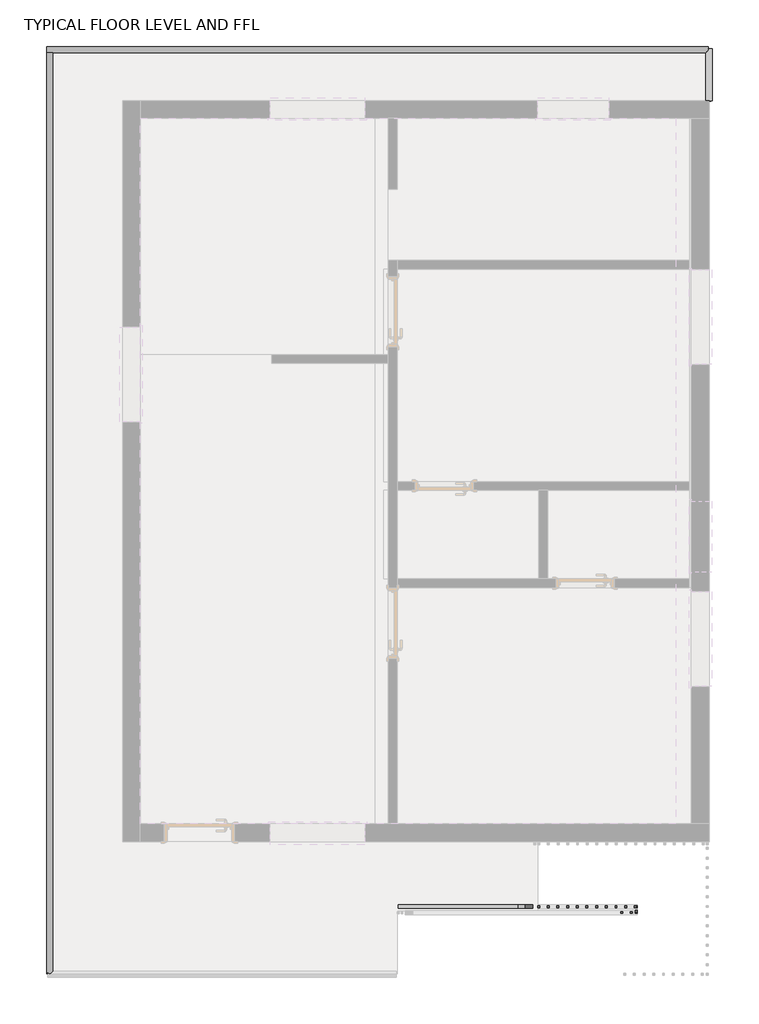
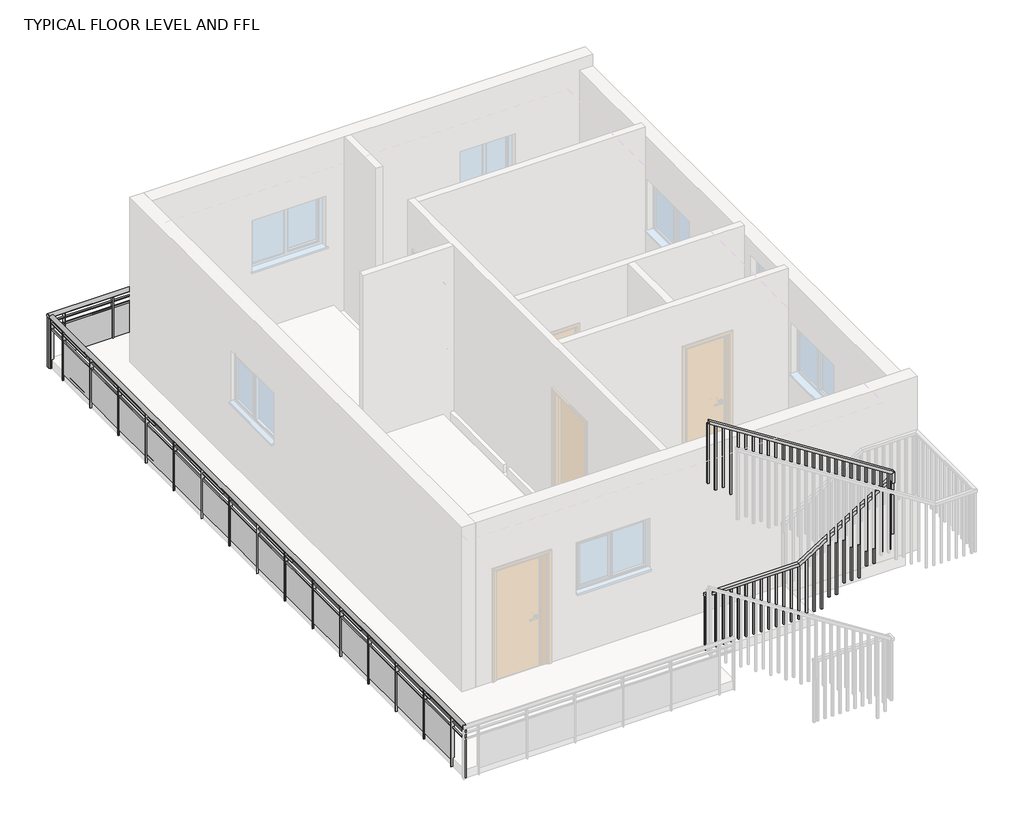
# One storey, part 3 of 3: 4 railings.
"""IFC4 building model written with IfcOpenShell, lengths in millimetres."""

from ifc_helpers import new_model, si_unit, point, frame, origin, place, context, project, spatial, polyline, ellipse_curve, trimmed, outline, extrude, faceted_brep, element, save
from ifc_brep_helpers import plane_surface, extruded_surface, advanced_brep

model = new_model("IFC4")

# Units and contexts
model_context = context("Model", 3, world=origin())
ifc_project = project(units=[si_unit("LENGTHUNIT", "METRE", prefix="MILLI")], contexts=[model_context])

# Site, building, storey
site = spatial("IfcSite", under=ifc_project)
building = spatial("IfcBuilding", under=site)
storey = spatial("IfcBuildingStorey", under=building, Name="TYPICAL FLOOR LEVEL AND FFL", Elevation=3535.68)

# Railings
placement = place(None, origin())
element("IfcRailing", 1, ObjectType="1100mm", at=placement, inside=storey, context=model_context, shape_type="SolidModel", body=[
    faceted_brep([(-10483.549573, -11032.9255223, 4676.32), (-10483.549573, -11032.9255223, 4626.32), (-10483.549573, -11082.9255223, 4626.32), (-10483.549573, -11082.9255223, 4676.32), (-8934.2055614, -11032.9255223, 4676.32), (-8919.5781391, -11032.9255223, 4626.32), (-8919.5781391, -11082.9255223, 4626.32), (-8934.2055614, -11082.9255223, 4676.32), (-7435.149573, -11032.9255223, 5635.5044027), (-7435.149573, -11082.9255223, 5635.5044027), (-7435.149573, -11082.9255223, 5576.1449155), (-7435.149573, -11032.9255223, 5576.1449155)], [[[0, 1, 2, 3]], [[1, 0, 4, 5]], [[2, 1, 5, 6]], [[3, 2, 6, 7]], [[0, 3, 7, 4]], [[8, 9, 10, 11]], [[5, 4, 8, 11]], [[6, 5, 11, 10]], [[7, 6, 10, 9]], [[4, 7, 9, 8]]]),
    faceted_brep([(-7385.149573, -11032.9255223, 5651.68), (-7385.149573, -11032.9255223, 5601.68), (-7435.149573, -11032.9255223, 5601.68), (-7435.149573, -11032.9255223, 5651.68), (-7385.149573, -11109.5255223, 5651.68), (-7435.149573, -11109.5255223, 5651.68), (-7435.149573, -11159.5255223, 5601.68), (-7385.149573, -11159.5255223, 5601.68)], [[[0, 1, 2, 3]], [[4, 5, 6, 7]], [[1, 0, 4, 7]], [[2, 1, 7, 6]], [[3, 2, 6, 5]], [[0, 3, 5, 4]]]),
    faceted_brep([(-7385.149573, -11109.5255223, 5651.68), (-7385.149573, -11159.5255223, 5601.68), (-7435.149573, -11159.5255223, 5601.68), (-7435.149573, -11109.5255223, 5651.68), (-7385.149573, -11109.5255223, 5798.3802481), (-7435.149573, -11109.5255223, 5771.0172146), (-7435.149573, -11159.5255223, 5771.0172146), (-7385.149573, -11159.5255223, 5798.3802481)], [[[0, 1, 2, 3]], [[4, 5, 6, 7]], [[1, 0, 4, 7]], [[2, 1, 7, 6]], [[3, 2, 6, 5]], [[0, 3, 5, 4]]]),
    faceted_brep([(-7385.149573, -11159.5255223, 5798.3802481), (-7435.149573, -11159.5255223, 5771.0172146), (-7435.149573, -11109.5255223, 5771.0172146), (-7385.149573, -11109.5255223, 5798.3802481), (-10457.8773536, -11159.5255223, 7764.96), (-10457.8773536, -11109.5255223, 7764.96), (-10457.8773536, -11109.5255223, 7705.5964137), (-10457.8773536, -11159.5255223, 7705.5964137)], [[[0, 1, 2, 3]], [[4, 5, 6, 7]], [[1, 0, 4, 7]], [[2, 1, 7, 6]], [[3, 2, 6, 5]], [[0, 3, 5, 4]]]),
    extrude(outline(polyline([(6664.96, -10460.149573), (7707.0506592, -10460.149573), (7723.0509356, -10485.149573), (6664.96, -10485.149573), (6664.96, -10460.149573)])), frame((0.0, -11147.0255223, 0.0), z_axis=(0.0, 1.0, 0.0), x_axis=(0.0, 0.0, 1.0)), (0.0, 0.0, 1.0), 25.0),
    extrude(outline(polyline([(6502.4, -10335.149573), (7627.0492772, -10335.149573), (7643.0495536, -10360.149573), (6502.4, -10360.149573), (6502.4, -10335.149573)])), frame((0.0, -11147.0255223, 0.0), z_axis=(0.0, 1.0, 0.0), x_axis=(0.0, 0.0, 1.0)), (0.0, 0.0, 1.0), 25.0),
    extrude(outline(polyline([(6502.4, -10210.149573), (7547.0478952, -10210.149573), (7563.0481716, -10235.149573), (6502.4, -10235.149573), (6502.4, -10210.149573)])), frame((0.0, -11147.0255223, 0.0), z_axis=(0.0, 1.0, 0.0), x_axis=(0.0, 0.0, 1.0)), (0.0, 0.0, 1.0), 25.0),
    extrude(outline(polyline([(6339.84, -10085.149573), (7467.0465132, -10085.149573), (7483.0467896, -10110.149573), (6339.84, -10110.149573), (6339.84, -10085.149573)])), frame((0.0, -11147.0255223, 0.0), z_axis=(0.0, 1.0, 0.0), x_axis=(0.0, 0.0, 1.0)), (0.0, 0.0, 1.0), 25.0),
    extrude(outline(polyline([(6339.84, -9960.149573), (7387.0451312, -9960.149573), (7403.0454076, -9985.149573), (6339.84, -9985.149573), (6339.84, -9960.149573)])), frame((0.0, -11147.0255223, 0.0), z_axis=(0.0, 1.0, 0.0), x_axis=(0.0, 0.0, 1.0)), (0.0, 0.0, 1.0), 25.0),
    extrude(outline(polyline([(6177.28, -9835.149573), (7307.0437492, -9835.149573), (7323.0440256, -9860.149573), (6177.28, -9860.149573), (6177.28, -9835.149573)])), frame((0.0, -11147.0255223, 0.0), z_axis=(0.0, 1.0, 0.0), x_axis=(0.0, 0.0, 1.0)), (0.0, 0.0, 1.0), 25.0),
    extrude(outline(polyline([(6177.28, -9710.149573), (7227.0423672, -9710.149573), (7243.0426436, -9735.149573), (6177.28, -9735.149573), (6177.28, -9710.149573)])), frame((0.0, -11147.0255223, 0.0), z_axis=(0.0, 1.0, 0.0), x_axis=(0.0, 0.0, 1.0)), (0.0, 0.0, 1.0), 25.0),
    extrude(outline(polyline([(6014.72, -9585.149573), (7147.0409852, -9585.149573), (7163.0412616, -9610.149573), (6014.72, -9610.149573), (6014.72, -9585.149573)])), frame((0.0, -11147.0255223, 0.0), z_axis=(0.0, 1.0, 0.0), x_axis=(0.0, 0.0, 1.0)), (0.0, 0.0, 1.0), 25.0),
    extrude(outline(polyline([(6014.72, -9460.149573), (7067.0396031, -9460.149573), (7083.0398795, -9485.149573), (6014.72, -9485.149573), (6014.72, -9460.149573)])), frame((0.0, -11147.0255223, 0.0), z_axis=(0.0, 1.0, 0.0), x_axis=(0.0, 0.0, 1.0)), (0.0, 0.0, 1.0), 25.0),
    extrude(outline(polyline([(5852.16, -9335.149573), (6987.0382211, -9335.149573), (7003.0384975, -9360.149573), (5852.16, -9360.149573), (5852.16, -9335.149573)])), frame((0.0, -11147.0255223, 0.0), z_axis=(0.0, 1.0, 0.0), x_axis=(0.0, 0.0, 1.0)), (0.0, 0.0, 1.0), 25.0),
    extrude(outline(polyline([(5852.16, -9210.149573), (6907.0368391, -9210.149573), (6923.0371155, -9235.149573), (5852.16, -9235.149573), (5852.16, -9210.149573)])), frame((0.0, -11147.0255223, 0.0), z_axis=(0.0, 1.0, 0.0), x_axis=(0.0, 0.0, 1.0)), (0.0, 0.0, 1.0), 25.0),
    extrude(outline(polyline([(5689.6, -9085.149573), (6827.0354571, -9085.149573), (6843.0357335, -9110.149573), (5689.6, -9110.149573), (5689.6, -9085.149573)])), frame((0.0, -11147.0255223, 0.0), z_axis=(0.0, 1.0, 0.0), x_axis=(0.0, 0.0, 1.0)), (0.0, 0.0, 1.0), 25.0),
    extrude(outline(polyline([(5689.6, -8960.149573), (6747.0340751, -8960.149573), (6763.0343515, -8985.149573), (5689.6, -8985.149573), (5689.6, -8960.149573)])), frame((0.0, -11147.0255223, 0.0), z_axis=(0.0, 1.0, 0.0), x_axis=(0.0, 0.0, 1.0)), (0.0, 0.0, 1.0), 25.0),
    extrude(outline(polyline([(5527.04, -8835.149573), (6667.0326931, -8835.149573), (6683.0329695, -8860.149573), (5527.04, -8860.149573), (5527.04, -8835.149573)])), frame((0.0, -11147.0255223, 0.0), z_axis=(0.0, 1.0, 0.0), x_axis=(0.0, 0.0, 1.0)), (0.0, 0.0, 1.0), 25.0),
    extrude(outline(polyline([(5527.04, -8710.149573), (6587.0313111, -8710.149573), (6603.0315875, -8735.149573), (5527.04, -8735.149573), (5527.04, -8710.149573)])), frame((0.0, -11147.0255223, 0.0), z_axis=(0.0, 1.0, 0.0), x_axis=(0.0, 0.0, 1.0)), (0.0, 0.0, 1.0), 25.0),
    extrude(outline(polyline([(5364.48, -8585.149573), (6507.0299291, -8585.149573), (6523.0302055, -8610.149573), (5364.48, -8610.149573), (5364.48, -8585.149573)])), frame((0.0, -11147.0255223, 0.0), z_axis=(0.0, 1.0, 0.0), x_axis=(0.0, 0.0, 1.0)), (0.0, 0.0, 1.0), 25.0),
    extrude(outline(polyline([(5364.48, -8460.149573), (6427.0285471, -8460.149573), (6443.0288235, -8485.149573), (5364.48, -8485.149573), (5364.48, -8460.149573)])), frame((0.0, -11147.0255223, 0.0), z_axis=(0.0, 1.0, 0.0), x_axis=(0.0, 0.0, 1.0)), (0.0, 0.0, 1.0), 25.0),
    extrude(outline(polyline([(5201.92, -8335.149573), (6347.0271651, -8335.149573), (6363.0274415, -8360.149573), (5201.92, -8360.149573), (5201.92, -8335.149573)])), frame((0.0, -11147.0255223, 0.0), z_axis=(0.0, 1.0, 0.0), x_axis=(0.0, 0.0, 1.0)), (0.0, 0.0, 1.0), 25.0),
    extrude(outline(polyline([(5201.92, -8210.149573), (6267.0257831, -8210.149573), (6283.0260595, -8235.149573), (5201.92, -8235.149573), (5201.92, -8210.149573)])), frame((0.0, -11147.0255223, 0.0), z_axis=(0.0, 1.0, 0.0), x_axis=(0.0, 0.0, 1.0)), (0.0, 0.0, 1.0), 25.0),
    extrude(outline(polyline([(5039.36, -8085.149573), (6187.024401, -8085.149573), (6203.0246774, -8110.149573), (5039.36, -8110.149573), (5039.36, -8085.149573)])), frame((0.0, -11147.0255223, 0.0), z_axis=(0.0, 1.0, 0.0), x_axis=(0.0, 0.0, 1.0)), (0.0, 0.0, 1.0), 25.0),
    extrude(outline(polyline([(5039.36, -7960.149573), (6107.023019, -7960.149573), (6123.0232954, -7985.149573), (5039.36, -7985.149573), (5039.36, -7960.149573)])), frame((0.0, -11147.0255223, 0.0), z_axis=(0.0, 1.0, 0.0), x_axis=(0.0, 0.0, 1.0)), (0.0, 0.0, 1.0), 25.0),
    extrude(outline(polyline([(4876.8, -7835.149573), (6027.021637, -7835.149573), (6043.0219134, -7860.149573), (4876.8, -7860.149573), (4876.8, -7835.149573)])), frame((0.0, -11147.0255223, 0.0), z_axis=(0.0, 1.0, 0.0), x_axis=(0.0, 0.0, 1.0)), (0.0, 0.0, 1.0), 25.0),
    extrude(outline(polyline([(4876.8, -7710.149573), (5947.020255, -7710.149573), (5963.0205314, -7735.149573), (4876.8, -7735.149573), (4876.8, -7710.149573)])), frame((0.0, -11147.0255223, 0.0), z_axis=(0.0, 1.0, 0.0), x_axis=(0.0, 0.0, 1.0)), (0.0, 0.0, 1.0), 25.0),
    extrude(outline(polyline([(4714.24, -7585.149573), (5867.018873, -7585.149573), (5883.0191494, -7610.149573), (4714.24, -7610.149573), (4714.24, -7585.149573)])), frame((0.0, -11147.0255223, 0.0), z_axis=(0.0, 1.0, 0.0), x_axis=(0.0, 0.0, 1.0)), (0.0, 0.0, 1.0), 25.0),
    extrude(outline(polyline([(4714.24, -7460.149573), (5787.017491, -7460.149573), (5803.0177674, -7485.149573), (4714.24, -7485.149573), (4714.24, -7460.149573)])), frame((0.0, -11147.0255223, 0.0), z_axis=(0.0, 1.0, 0.0), x_axis=(0.0, 0.0, 1.0)), (0.0, 0.0, 1.0), 25.0),
    extrude(outline(polyline([(-7422.649573, -11107.9255223), (-7397.649573, -11107.9255223), (-7397.649573, -11132.9255223), (-7422.649573, -11132.9255223), (-7422.649573, -11107.9255223)])), frame((0.0, 0.0, 4701.5601967), z_axis=(0.0, 0.0, 1.0), x_axis=(1.0, 0.0, 0.0)), (0.0, 0.0, 1.0), 900.1198033),
    extrude(outline(polyline([(5577.1686899, -7433.549573), (4389.12, -7433.549573), (4389.12, -7408.549573), (5593.1651638, -7408.549573), (5577.1686899, -7433.549573)])), frame((0.0, -11070.4255223, 0.0), z_axis=(0.0, 1.0, 0.0), x_axis=(0.0, 0.0, 1.0)), (0.0, 0.0, 1.0), 25.0),
    extrude(outline(polyline([(5497.1863201, -7558.549573), (4389.12, -7558.549573), (4389.12, -7533.549573), (5513.1827941, -7533.549573), (5497.1863201, -7558.549573)])), frame((0.0, -11070.4255223, 0.0), z_axis=(0.0, 1.0, 0.0), x_axis=(0.0, 0.0, 1.0)), (0.0, 0.0, 1.0), 25.0),
    extrude(outline(polyline([(5417.2039504, -7683.549573), (4226.56, -7683.549573), (4226.56, -7658.549573), (5433.2004243, -7658.549573), (5417.2039504, -7683.549573)])), frame((0.0, -11070.4255223, 0.0), z_axis=(0.0, 1.0, 0.0), x_axis=(0.0, 0.0, 1.0)), (0.0, 0.0, 1.0), 25.0),
    extrude(outline(polyline([(5337.2215806, -7808.549573), (4226.56, -7808.549573), (4226.56, -7783.549573), (5353.2180546, -7783.549573), (5337.2215806, -7808.549573)])), frame((0.0, -11070.4255223, 0.0), z_axis=(0.0, 1.0, 0.0), x_axis=(0.0, 0.0, 1.0)), (0.0, 0.0, 1.0), 25.0),
    extrude(outline(polyline([(5257.2392109, -7933.549573), (4064.0, -7933.549573), (4064.0, -7908.549573), (5273.2356848, -7908.549573), (5257.2392109, -7933.549573)])), frame((0.0, -11070.4255223, 0.0), z_axis=(0.0, 1.0, 0.0), x_axis=(0.0, 0.0, 1.0)), (0.0, 0.0, 1.0), 25.0),
    extrude(outline(polyline([(5177.2568411, -8058.549573), (4064.0, -8058.549573), (4064.0, -8033.549573), (5193.2533151, -8033.549573), (5177.2568411, -8058.549573)])), frame((0.0, -11070.4255223, 0.0), z_axis=(0.0, 1.0, 0.0), x_axis=(0.0, 0.0, 1.0)), (0.0, 0.0, 1.0), 25.0),
    extrude(outline(polyline([(5097.2744714, -8183.549573), (4064.0, -8183.549573), (4064.0, -8158.549573), (5113.2709453, -8158.549573), (5097.2744714, -8183.549573)])), frame((0.0, -11070.4255223, 0.0), z_axis=(0.0, 1.0, 0.0), x_axis=(0.0, 0.0, 1.0)), (0.0, 0.0, 1.0), 25.0),
    extrude(outline(polyline([(5017.2921016, -8308.549573), (3901.44, -8308.549573), (3901.44, -8283.549573), (5033.2885756, -8283.549573), (5017.2921016, -8308.549573)])), frame((0.0, -11070.4255223, 0.0), z_axis=(0.0, 1.0, 0.0), x_axis=(0.0, 0.0, 1.0)), (0.0, 0.0, 1.0), 25.0),
    extrude(outline(polyline([(4937.3097319, -8433.549573), (3901.44, -8433.549573), (3901.44, -8408.549573), (4953.3062058, -8408.549573), (4937.3097319, -8433.549573)])), frame((0.0, -11070.4255223, 0.0), z_axis=(0.0, 1.0, 0.0), x_axis=(0.0, 0.0, 1.0)), (0.0, 0.0, 1.0), 25.0),
    extrude(outline(polyline([(4857.3273621, -8558.549573), (3738.88, -8558.549573), (3738.88, -8533.549573), (4873.3238361, -8533.549573), (4857.3273621, -8558.549573)])), frame((0.0, -11070.4255223, 0.0), z_axis=(0.0, 1.0, 0.0), x_axis=(0.0, 0.0, 1.0)), (0.0, 0.0, 1.0), 25.0),
    extrude(outline(polyline([(4777.3449924, -8683.549573), (3738.88, -8683.549573), (3738.88, -8658.549573), (4793.3414663, -8658.549573), (4777.3449924, -8683.549573)])), frame((0.0, -11070.4255223, 0.0), z_axis=(0.0, 1.0, 0.0), x_axis=(0.0, 0.0, 1.0)), (0.0, 0.0, 1.0), 25.0),
    extrude(outline(polyline([(4697.3626226, -8808.549573), (3664.7203468, -8808.549573), (3664.7203468, -8783.549573), (4713.3590966, -8783.549573), (4697.3626226, -8808.549573)])), frame((0.0, -11070.4255223, 0.0), z_axis=(0.0, 1.0, 0.0), x_axis=(0.0, 0.0, 1.0)), (0.0, 0.0, 1.0), 25.0),
    extrude(outline(polyline([(4617.3802529, -8933.549573), (3584.737977, -8933.549573), (3584.737977, -8908.549573), (4633.3767268, -8908.549573), (4617.3802529, -8933.549573)])), frame((0.0, -11070.4255223, 0.0), z_axis=(0.0, 1.0, 0.0), x_axis=(0.0, 0.0, 1.0)), (0.0, 0.0, 1.0), 25.0),
    extrude(outline(polyline([(-9058.549573, -11070.4255223), (-9058.549573, -11045.4255223), (-9033.549573, -11045.4255223), (-9033.549573, -11070.4255223), (-9058.549573, -11070.4255223)])), frame((0.0, 0.0, 3576.32), z_axis=(0.0, 0.0, 1.0), x_axis=(1.0, 0.0, 0.0)), (0.0, 0.0, 1.0), 1050.0),
    extrude(outline(polyline([(-9183.549573, -11070.4255223), (-9183.549573, -11045.4255223), (-9158.549573, -11045.4255223), (-9158.549573, -11070.4255223), (-9183.549573, -11070.4255223)])), frame((0.0, 0.0, 3576.32), z_axis=(0.0, 0.0, 1.0), x_axis=(1.0, 0.0, 0.0)), (0.0, 0.0, 1.0), 1050.0),
    extrude(outline(polyline([(-9308.549573, -11070.4255223), (-9308.549573, -11045.4255223), (-9283.549573, -11045.4255223), (-9283.549573, -11070.4255223), (-9308.549573, -11070.4255223)])), frame((0.0, 0.0, 3576.32), z_axis=(0.0, 0.0, 1.0), x_axis=(1.0, 0.0, 0.0)), (0.0, 0.0, 1.0), 1050.0),
    extrude(outline(polyline([(-9433.549573, -11070.4255223), (-9433.549573, -11045.4255223), (-9408.549573, -11045.4255223), (-9408.549573, -11070.4255223), (-9433.549573, -11070.4255223)])), frame((0.0, 0.0, 3576.32), z_axis=(0.0, 0.0, 1.0), x_axis=(1.0, 0.0, 0.0)), (0.0, 0.0, 1.0), 1050.0),
    extrude(outline(polyline([(-9558.549573, -11070.4255223), (-9558.549573, -11045.4255223), (-9533.549573, -11045.4255223), (-9533.549573, -11070.4255223), (-9558.549573, -11070.4255223)])), frame((0.0, 0.0, 3576.32), z_axis=(0.0, 0.0, 1.0), x_axis=(1.0, 0.0, 0.0)), (0.0, 0.0, 1.0), 1050.0),
    extrude(outline(polyline([(-9683.549573, -11070.4255223), (-9683.549573, -11045.4255223), (-9658.549573, -11045.4255223), (-9658.549573, -11070.4255223), (-9683.549573, -11070.4255223)])), frame((0.0, 0.0, 3576.32), z_axis=(0.0, 0.0, 1.0), x_axis=(1.0, 0.0, 0.0)), (0.0, 0.0, 1.0), 1050.0),
    extrude(outline(polyline([(-9808.549573, -11070.4255223), (-9808.549573, -11045.4255223), (-9783.549573, -11045.4255223), (-9783.549573, -11070.4255223), (-9808.549573, -11070.4255223)])), frame((0.0, 0.0, 3576.32), z_axis=(0.0, 0.0, 1.0), x_axis=(1.0, 0.0, 0.0)), (0.0, 0.0, 1.0), 1050.0),
    extrude(outline(polyline([(-9933.549573, -11070.4255223), (-9933.549573, -11045.4255223), (-9908.549573, -11045.4255223), (-9908.549573, -11070.4255223), (-9933.549573, -11070.4255223)])), frame((0.0, 0.0, 3576.32), z_axis=(0.0, 0.0, 1.0), x_axis=(1.0, 0.0, 0.0)), (0.0, 0.0, 1.0), 1050.0),
    extrude(outline(polyline([(-10058.549573, -11070.4255223), (-10058.549573, -11045.4255223), (-10033.549573, -11045.4255223), (-10033.549573, -11070.4255223), (-10058.549573, -11070.4255223)])), frame((0.0, 0.0, 3576.32), z_axis=(0.0, 0.0, 1.0), x_axis=(1.0, 0.0, 0.0)), (0.0, 0.0, 1.0), 1050.0),
    extrude(outline(polyline([(-10183.549573, -11070.4255223), (-10183.549573, -11045.4255223), (-10158.549573, -11045.4255223), (-10158.549573, -11070.4255223), (-10183.549573, -11070.4255223)])), frame((0.0, 0.0, 3576.32), z_axis=(0.0, 0.0, 1.0), x_axis=(1.0, 0.0, 0.0)), (0.0, 0.0, 1.0), 1050.0),
    extrude(outline(polyline([(-10308.549573, -11070.4255223), (-10308.549573, -11045.4255223), (-10283.549573, -11045.4255223), (-10283.549573, -11070.4255223), (-10308.549573, -11070.4255223)])), frame((0.0, 0.0, 3576.32), z_axis=(0.0, 0.0, 1.0), x_axis=(1.0, 0.0, 0.0)), (0.0, 0.0, 1.0), 1050.0),
    extrude(outline(polyline([(-10433.549573, -11070.4255223), (-10433.549573, -11045.4255223), (-10408.549573, -11045.4255223), (-10408.549573, -11070.4255223), (-10433.549573, -11070.4255223)])), frame((0.0, 0.0, 3576.32), z_axis=(0.0, 0.0, 1.0), x_axis=(1.0, 0.0, 0.0)), (0.0, 0.0, 1.0), 1050.0),
    extrude(outline(polyline([(-7422.649573, -11122.0255223), (-7397.649573, -11122.0255223), (-7397.649573, -11147.0255223), (-7422.649573, -11147.0255223), (-7422.649573, -11122.0255223)])), frame((0.0, 0.0, 4701.5601967), z_axis=(0.0, 0.0, 1.0), x_axis=(1.0, 0.0, 0.0)), (0.0, 0.0, 1.0), 900.1198033),
    extrude(outline(polyline([(5584.1431525, -7422.649573), (4389.12, -7422.649573), (4389.12, -7397.649573), (5600.1396265, -7397.649573), (5584.1431525, -7422.649573)])), frame((0.0, -11070.4255223, 0.0), z_axis=(0.0, 1.0, 0.0), x_axis=(0.0, 0.0, 1.0)), (0.0, 0.0, 1.0), 25.0),
    extrude(outline(polyline([(6664.96, -10458.549573), (7706.0266415, -10458.549573), (7722.0269179, -10483.549573), (6664.96, -10483.549573), (6664.96, -10458.549573)])), frame((0.0, -11147.0255223, 0.0), z_axis=(0.0, 1.0, 0.0), x_axis=(0.0, 0.0, 1.0)), (0.0, 0.0, 1.0), 25.0),
    extrude(outline(polyline([(-10483.549573, -11070.4255223), (-10483.549573, -11045.4255223), (-10458.549573, -11045.4255223), (-10458.549573, -11070.4255223), (-10483.549573, -11070.4255223)])), frame((0.0, 0.0, 3576.32), z_axis=(0.0, 0.0, 1.0), x_axis=(1.0, 0.0, 0.0)), (0.0, 0.0, 1.0), 1050.0),
])
element("IfcRailing", 2, ObjectType="Glass_Panel-Bottom_Fill", at=placement, inside=storey, context=model_context, shape_type="SolidModel", body=[
    advanced_brep(
    [(-15017.4420435, 42.847874, 4435.68), (-15017.4420435, -37.152126, 4435.68), (-6483.0420435, 42.847874, 4435.68), (-6483.0420435, -37.152126, 4435.68)],
    [
        (0, 1, ellipse_curve(frame((-15017.4420435, 2.847874, 4435.68), z_axis=(-1.0, 0.0, 0.0), x_axis=(0.0, -1.0, 0.0)), 40.0, 30.0)),
        (1, 0, ellipse_curve(frame((-15017.4420435, 2.847874, 4435.68), z_axis=(-1.0, 0.0, 0.0), x_axis=(0.0, -1.0, 0.0)), 40.0, 30.0)),
        (2, 3, ellipse_curve(frame((-6483.0420435, 2.847874, 4435.68), z_axis=(1.0, 0.0, 0.0), x_axis=(0.0, -1.0, 0.0)), 40.0, 30.0)),
        (3, 2, ellipse_curve(frame((-6483.0420435, 2.847874, 4435.68), z_axis=(1.0, 0.0, 0.0), x_axis=(0.0, -1.0, 0.0)), 40.0, 30.0)),
        (0, 2),
        (3, 1),
    ],
    [
        plane_surface(frame((-15017.4420435, 2.847874, 4435.68), z_axis=(-1.0, 0.0, 0.0), x_axis=(0.0, 1.0, 0.0))),
        plane_surface(frame((-6483.0420435, 2.847874, 4435.68), z_axis=(1.0, 0.0, 0.0), x_axis=(0.0, 1.0, 0.0))),
        extruded_surface(trimmed(ellipse_curve(frame((-6483.0420435, 2.847874, 4435.68), z_axis=(-1.0, 0.0, 0.0), x_axis=(0.0, -1.0, 0.0)), 40.0, 30.0), [point((-6483.0420435, 42.847874, 4435.68))], [point((-6483.0420435, -37.152126, 4435.68))], True, "CARTESIAN"), (-8534.4, 0.0, 0.0), 8534.4),
        extruded_surface(trimmed(ellipse_curve(frame((-6483.0420435, 2.847874, 4435.68), z_axis=(-1.0, 0.0, 0.0), x_axis=(0.0, -1.0, 0.0)), 40.0, 30.0), [point((-6483.0420435, -37.152126, 4435.68))], [point((-6483.0420435, 42.847874, 4435.68))], True, "CARTESIAN"), (-8534.4, 0.0, 0.0), 8534.4),
    ],
    [
        (0, [[1, 2]]),
        (1, [[3, 4]]),
        (2, [[-1, 5, -4, 6]]),
        (3, [[-2, -6, -3, -5]]),
    ],
),
    extrude(outline(polyline([(-15017.4420435, -6.5428911), (-15017.4420435, 13.4571089), (-6483.0420435, 13.4571089), (-6483.0420435, -6.5428911), (-15017.4420435, -6.5428911)])), frame((0.0, 0.0, 4315.68), z_axis=(0.0, 0.0, 1.0), x_axis=(1.0, 0.0, 0.0)), (0.0, 0.0, 1.0), 20.0),
    extrude(outline(polyline([(-15017.4420435, -6.5428911), (-15017.4420435, 13.4571089), (-6483.0420435, 13.4571089), (-6483.0420435, -6.5428911), (-15017.4420435, -6.5428911)])), frame((0.0, 0.0, 4215.68), z_axis=(0.0, 0.0, 1.0), x_axis=(1.0, 0.0, 0.0)), (0.0, 0.0, 1.0), 20.0),
    extrude(outline(polyline([(-6756.2420435, 28.4571089), (-6744.2420435, 28.4571089), (-6744.2420435, -21.5428911), (-6756.2420435, -21.5428911), (-6756.2420435, 28.4571089)])), frame((0.0, 0.0, 3535.68), z_axis=(0.0, 0.0, 1.0), x_axis=(1.0, 0.0, 0.0)), (0.0, 0.0, 1.0), 870.0),
    extrude(outline(polyline([(-7550.2420435, 1.7322988), (-6750.2420435, 1.7322988), (-6750.2420435, -3.2677012), (-7550.2420435, -3.2677012), (-7550.2420435, 1.7322988)])), frame((0.0, 0.0, 3635.68), z_axis=(0.0, 0.0, 1.0), x_axis=(1.0, 0.0, 0.0)), (0.0, 0.0, 1.0), 580.0),
    extrude(outline(polyline([(-7556.2420435, 28.4571089), (-7544.2420435, 28.4571089), (-7544.2420435, -21.5428911), (-7556.2420435, -21.5428911), (-7556.2420435, 28.4571089)])), frame((0.0, 0.0, 3535.68), z_axis=(0.0, 0.0, 1.0), x_axis=(1.0, 0.0, 0.0)), (0.0, 0.0, 1.0), 870.0),
    extrude(outline(polyline([(-8350.2420435, 1.7322988), (-7550.2420435, 1.7322988), (-7550.2420435, -3.2677012), (-8350.2420435, -3.2677012), (-8350.2420435, 1.7322988)])), frame((0.0, 0.0, 3635.68), z_axis=(0.0, 0.0, 1.0), x_axis=(1.0, 0.0, 0.0)), (0.0, 0.0, 1.0), 580.0),
    extrude(outline(polyline([(-8356.2420435, 28.4571089), (-8344.2420435, 28.4571089), (-8344.2420435, -21.5428911), (-8356.2420435, -21.5428911), (-8356.2420435, 28.4571089)])), frame((0.0, 0.0, 3535.68), z_axis=(0.0, 0.0, 1.0), x_axis=(1.0, 0.0, 0.0)), (0.0, 0.0, 1.0), 870.0),
    extrude(outline(polyline([(-9150.2420435, 1.7322988), (-8350.2420435, 1.7322988), (-8350.2420435, -3.2677012), (-9150.2420435, -3.2677012), (-9150.2420435, 1.7322988)])), frame((0.0, 0.0, 3635.68), z_axis=(0.0, 0.0, 1.0), x_axis=(1.0, 0.0, 0.0)), (0.0, 0.0, 1.0), 580.0),
    extrude(outline(polyline([(-9156.2420435, 28.4571089), (-9144.2420435, 28.4571089), (-9144.2420435, -21.5428911), (-9156.2420435, -21.5428911), (-9156.2420435, 28.4571089)])), frame((0.0, 0.0, 3535.68), z_axis=(0.0, 0.0, 1.0), x_axis=(1.0, 0.0, 0.0)), (0.0, 0.0, 1.0), 870.0),
    extrude(outline(polyline([(-9950.2420435, 1.7322988), (-9150.2420435, 1.7322988), (-9150.2420435, -3.2677012), (-9950.2420435, -3.2677012), (-9950.2420435, 1.7322988)])), frame((0.0, 0.0, 3635.68), z_axis=(0.0, 0.0, 1.0), x_axis=(1.0, 0.0, 0.0)), (0.0, 0.0, 1.0), 580.0),
    extrude(outline(polyline([(-9956.2420435, 28.4571089), (-9944.2420435, 28.4571089), (-9944.2420435, -21.5428911), (-9956.2420435, -21.5428911), (-9956.2420435, 28.4571089)])), frame((0.0, 0.0, 3535.68), z_axis=(0.0, 0.0, 1.0), x_axis=(1.0, 0.0, 0.0)), (0.0, 0.0, 1.0), 870.0),
    extrude(outline(polyline([(-10750.2420435, 1.7322988), (-9950.2420435, 1.7322988), (-9950.2420435, -3.2677012), (-10750.2420435, -3.2677012), (-10750.2420435, 1.7322988)])), frame((0.0, 0.0, 3635.68), z_axis=(0.0, 0.0, 1.0), x_axis=(1.0, 0.0, 0.0)), (0.0, 0.0, 1.0), 580.0),
    extrude(outline(polyline([(-10756.2420435, 28.4571089), (-10744.2420435, 28.4571089), (-10744.2420435, -21.5428911), (-10756.2420435, -21.5428911), (-10756.2420435, 28.4571089)])), frame((0.0, 0.0, 3535.68), z_axis=(0.0, 0.0, 1.0), x_axis=(1.0, 0.0, 0.0)), (0.0, 0.0, 1.0), 870.0),
    extrude(outline(polyline([(-11550.2420435, 1.7322988), (-10750.2420435, 1.7322988), (-10750.2420435, -3.2677012), (-11550.2420435, -3.2677012), (-11550.2420435, 1.7322988)])), frame((0.0, 0.0, 3635.68), z_axis=(0.0, 0.0, 1.0), x_axis=(1.0, 0.0, 0.0)), (0.0, 0.0, 1.0), 580.0),
    extrude(outline(polyline([(-11556.2420435, 28.4571089), (-11544.2420435, 28.4571089), (-11544.2420435, -21.5428911), (-11556.2420435, -21.5428911), (-11556.2420435, 28.4571089)])), frame((0.0, 0.0, 3535.68), z_axis=(0.0, 0.0, 1.0), x_axis=(1.0, 0.0, 0.0)), (0.0, 0.0, 1.0), 870.0),
    extrude(outline(polyline([(-12350.2420435, 1.7322988), (-11550.2420435, 1.7322988), (-11550.2420435, -3.2677012), (-12350.2420435, -3.2677012), (-12350.2420435, 1.7322988)])), frame((0.0, 0.0, 3635.68), z_axis=(0.0, 0.0, 1.0), x_axis=(1.0, 0.0, 0.0)), (0.0, 0.0, 1.0), 580.0),
    extrude(outline(polyline([(-12356.2420435, 28.4571089), (-12344.2420435, 28.4571089), (-12344.2420435, -21.5428911), (-12356.2420435, -21.5428911), (-12356.2420435, 28.4571089)])), frame((0.0, 0.0, 3535.68), z_axis=(0.0, 0.0, 1.0), x_axis=(1.0, 0.0, 0.0)), (0.0, 0.0, 1.0), 870.0),
    extrude(outline(polyline([(-13150.2420435, 1.7322988), (-12350.2420435, 1.7322988), (-12350.2420435, -3.2677012), (-13150.2420435, -3.2677012), (-13150.2420435, 1.7322988)])), frame((0.0, 0.0, 3635.68), z_axis=(0.0, 0.0, 1.0), x_axis=(1.0, 0.0, 0.0)), (0.0, 0.0, 1.0), 580.0),
    extrude(outline(polyline([(-13156.2420435, 28.4571089), (-13144.2420435, 28.4571089), (-13144.2420435, -21.5428911), (-13156.2420435, -21.5428911), (-13156.2420435, 28.4571089)])), frame((0.0, 0.0, 3535.68), z_axis=(0.0, 0.0, 1.0), x_axis=(1.0, 0.0, 0.0)), (0.0, 0.0, 1.0), 870.0),
    extrude(outline(polyline([(-13950.2420435, 1.7322988), (-13150.2420435, 1.7322988), (-13150.2420435, -3.2677012), (-13950.2420435, -3.2677012), (-13950.2420435, 1.7322988)])), frame((0.0, 0.0, 3635.68), z_axis=(0.0, 0.0, 1.0), x_axis=(1.0, 0.0, 0.0)), (0.0, 0.0, 1.0), 580.0),
    extrude(outline(polyline([(-13956.2420435, 28.4571089), (-13944.2420435, 28.4571089), (-13944.2420435, -21.5428911), (-13956.2420435, -21.5428911), (-13956.2420435, 28.4571089)])), frame((0.0, 0.0, 3535.68), z_axis=(0.0, 0.0, 1.0), x_axis=(1.0, 0.0, 0.0)), (0.0, 0.0, 1.0), 870.0),
    extrude(outline(polyline([(-14750.2420435, 1.7322988), (-13950.2420435, 1.7322988), (-13950.2420435, -3.2677012), (-14750.2420435, -3.2677012), (-14750.2420435, 1.7322988)])), frame((0.0, 0.0, 3635.68), z_axis=(0.0, 0.0, 1.0), x_axis=(1.0, 0.0, 0.0)), (0.0, 0.0, 1.0), 580.0),
    extrude(outline(polyline([(-14756.2420435, 28.4571089), (-14744.2420435, 28.4571089), (-14744.2420435, -21.5428911), (-14756.2420435, -21.5428911), (-14756.2420435, 28.4571089)])), frame((0.0, 0.0, 3535.68), z_axis=(0.0, 0.0, 1.0), x_axis=(1.0, 0.0, 0.0)), (0.0, 0.0, 1.0), 870.0),
    extrude(outline(polyline([(-6491.0420435, 28.4571089), (-6479.0420435, 28.4571089), (-6479.0420435, -21.5428911), (-6491.0420435, -21.5428911), (-6491.0420435, 28.4571089)])), frame((0.0, 0.0, 3535.68), z_axis=(0.0, 0.0, 1.0), x_axis=(1.0, 0.0, 0.0)), (0.0, 0.0, 1.0), 870.0),
    extrude(outline(polyline([(-15021.4420435, 28.4571089), (-15009.4420435, 28.4571089), (-15009.4420435, -21.5428911), (-15021.4420435, -21.5428911), (-15021.4420435, 28.4571089)])), frame((0.0, 0.0, 3535.68), z_axis=(0.0, 0.0, 1.0), x_axis=(1.0, 0.0, 0.0)), (0.0, 0.0, 1.0), 870.0),
])
element("IfcRailing", 3, ObjectType="Glass_Panel-Bottom_Fill", at=placement, inside=storey, context=model_context, shape_type="SolidModel", body=[
    advanced_brep(
    [(-14939.9512783, -37.152126, 4435.68), (-15019.9512783, -37.152126, 4435.68), (-14939.9512783, -11928.1928911, 4435.68), (-15019.9512783, -11928.1928911, 4435.68)],
    [
        (0, 1, ellipse_curve(frame((-14979.9512783, -37.152126, 4435.68), z_axis=(0.0, 1.0, 0.0), x_axis=(-1.0, 0.0, 0.0)), 40.0, 30.0)),
        (1, 0, ellipse_curve(frame((-14979.9512783, -37.152126, 4435.68), z_axis=(0.0, 1.0, 0.0), x_axis=(-1.0, 0.0, 0.0)), 40.0, 30.0)),
        (2, 3, ellipse_curve(frame((-14979.9512783, -11928.1928911, 4435.68), z_axis=(0.0, -1.0, 0.0), x_axis=(-1.0, 0.0, 0.0)), 40.0, 30.0)),
        (3, 2, ellipse_curve(frame((-14979.9512783, -11928.1928911, 4435.68), z_axis=(0.0, -1.0, 0.0), x_axis=(-1.0, 0.0, 0.0)), 40.0, 30.0)),
        (0, 2),
        (3, 1),
    ],
    [
        plane_surface(frame((-14979.9512783, -37.152126, 4435.68), z_axis=(0.0, 1.0, 0.0), x_axis=(0.0, 0.0, -1.0))),
        plane_surface(frame((-14979.9512783, -11928.1928911, 4435.68), z_axis=(0.0, -1.0, 0.0), x_axis=(0.0, 0.0, -1.0))),
        extruded_surface(trimmed(ellipse_curve(frame((-14979.9512783, -11928.1928911, 4435.68), z_axis=(0.0, 1.0, 0.0), x_axis=(-1.0, 0.0, 0.0)), 40.0, 30.0), [point((-14939.9512783, -11928.1928911, 4435.68))], [point((-15019.9512783, -11928.1928911, 4435.68))], True, "CARTESIAN"), (0.0, 11891.040765099999, 0.0), 11891.040765099999),
        extruded_surface(trimmed(ellipse_curve(frame((-14979.9512783, -11928.1928911, 4435.68), z_axis=(0.0, 1.0, 0.0), x_axis=(-1.0, 0.0, 0.0)), 40.0, 30.0), [point((-15019.9512783, -11928.1928911, 4435.68))], [point((-14939.9512783, -11928.1928911, 4435.68))], True, "CARTESIAN"), (0.0, 11891.040765099999, 0.0), 11891.040765099999),
    ],
    [
        (0, [[1, 2]]),
        (1, [[3, 4]]),
        (2, [[-1, 5, -4, 6]]),
        (3, [[-2, -6, -3, -5]]),
    ],
),
    extrude(outline(polyline([(-14989.3420435, -37.152126), (-14969.3420435, -37.152126), (-14969.3420435, -11928.1928911), (-14989.3420435, -11928.1928911), (-14989.3420435, -37.152126)])), frame((0.0, 0.0, 4315.68), z_axis=(0.0, 0.0, 1.0), x_axis=(1.0, 0.0, 0.0)), (0.0, 0.0, 1.0), 20.0),
    extrude(outline(polyline([(-14989.3420435, -37.152126), (-14969.3420435, -37.152126), (-14969.3420435, -11928.1928911), (-14989.3420435, -11928.1928911), (-14989.3420435, -37.152126)])), frame((0.0, 0.0, 4215.68), z_axis=(0.0, 0.0, 1.0), x_axis=(1.0, 0.0, 0.0)), (0.0, 0.0, 1.0), 20.0),
    extrude(outline(polyline([(-14954.3420435, -11576.6725086), (-14954.3420435, -11588.6725086), (-15004.3420435, -11588.6725086), (-15004.3420435, -11576.6725086), (-14954.3420435, -11576.6725086)])), frame((0.0, 0.0, 3535.68), z_axis=(0.0, 0.0, 1.0), x_axis=(1.0, 0.0, 0.0)), (0.0, 0.0, 1.0), 870.0),
    extrude(outline(polyline([(-14981.0668536, -10782.6725086), (-14981.0668536, -11582.6725086), (-14986.0668536, -11582.6725086), (-14986.0668536, -10782.6725086), (-14981.0668536, -10782.6725086)])), frame((0.0, 0.0, 3635.68), z_axis=(0.0, 0.0, 1.0), x_axis=(1.0, 0.0, 0.0)), (0.0, 0.0, 1.0), 580.0),
    extrude(outline(polyline([(-14954.3420435, -10776.6725086), (-14954.3420435, -10788.6725086), (-15004.3420435, -10788.6725086), (-15004.3420435, -10776.6725086), (-14954.3420435, -10776.6725086)])), frame((0.0, 0.0, 3535.68), z_axis=(0.0, 0.0, 1.0), x_axis=(1.0, 0.0, 0.0)), (0.0, 0.0, 1.0), 870.0),
    extrude(outline(polyline([(-14981.0668536, -9982.6725086), (-14981.0668536, -10782.6725086), (-14986.0668536, -10782.6725086), (-14986.0668536, -9982.6725086), (-14981.0668536, -9982.6725086)])), frame((0.0, 0.0, 3635.68), z_axis=(0.0, 0.0, 1.0), x_axis=(1.0, 0.0, 0.0)), (0.0, 0.0, 1.0), 580.0),
    extrude(outline(polyline([(-14954.3420435, -9976.6725086), (-14954.3420435, -9988.6725086), (-15004.3420435, -9988.6725086), (-15004.3420435, -9976.6725086), (-14954.3420435, -9976.6725086)])), frame((0.0, 0.0, 3535.68), z_axis=(0.0, 0.0, 1.0), x_axis=(1.0, 0.0, 0.0)), (0.0, 0.0, 1.0), 870.0),
    extrude(outline(polyline([(-14981.0668536, -9182.6725086), (-14981.0668536, -9982.6725086), (-14986.0668536, -9982.6725086), (-14986.0668536, -9182.6725086), (-14981.0668536, -9182.6725086)])), frame((0.0, 0.0, 3635.68), z_axis=(0.0, 0.0, 1.0), x_axis=(1.0, 0.0, 0.0)), (0.0, 0.0, 1.0), 580.0),
    extrude(outline(polyline([(-14954.3420435, -9176.6725086), (-14954.3420435, -9188.6725086), (-15004.3420435, -9188.6725086), (-15004.3420435, -9176.6725086), (-14954.3420435, -9176.6725086)])), frame((0.0, 0.0, 3535.68), z_axis=(0.0, 0.0, 1.0), x_axis=(1.0, 0.0, 0.0)), (0.0, 0.0, 1.0), 870.0),
    extrude(outline(polyline([(-14981.0668536, -8382.6725086), (-14981.0668536, -9182.6725086), (-14986.0668536, -9182.6725086), (-14986.0668536, -8382.6725086), (-14981.0668536, -8382.6725086)])), frame((0.0, 0.0, 3635.68), z_axis=(0.0, 0.0, 1.0), x_axis=(1.0, 0.0, 0.0)), (0.0, 0.0, 1.0), 580.0),
    extrude(outline(polyline([(-14954.3420435, -8376.6725086), (-14954.3420435, -8388.6725086), (-15004.3420435, -8388.6725086), (-15004.3420435, -8376.6725086), (-14954.3420435, -8376.6725086)])), frame((0.0, 0.0, 3535.68), z_axis=(0.0, 0.0, 1.0), x_axis=(1.0, 0.0, 0.0)), (0.0, 0.0, 1.0), 870.0),
    extrude(outline(polyline([(-14981.0668536, -7582.6725086), (-14981.0668536, -8382.6725086), (-14986.0668536, -8382.6725086), (-14986.0668536, -7582.6725086), (-14981.0668536, -7582.6725086)])), frame((0.0, 0.0, 3635.68), z_axis=(0.0, 0.0, 1.0), x_axis=(1.0, 0.0, 0.0)), (0.0, 0.0, 1.0), 580.0),
    extrude(outline(polyline([(-14954.3420435, -7576.6725086), (-14954.3420435, -7588.6725086), (-15004.3420435, -7588.6725086), (-15004.3420435, -7576.6725086), (-14954.3420435, -7576.6725086)])), frame((0.0, 0.0, 3535.68), z_axis=(0.0, 0.0, 1.0), x_axis=(1.0, 0.0, 0.0)), (0.0, 0.0, 1.0), 870.0),
    extrude(outline(polyline([(-14981.0668536, -6782.6725086), (-14981.0668536, -7582.6725086), (-14986.0668536, -7582.6725086), (-14986.0668536, -6782.6725086), (-14981.0668536, -6782.6725086)])), frame((0.0, 0.0, 3635.68), z_axis=(0.0, 0.0, 1.0), x_axis=(1.0, 0.0, 0.0)), (0.0, 0.0, 1.0), 580.0),
    extrude(outline(polyline([(-14954.3420435, -6776.6725086), (-14954.3420435, -6788.6725086), (-15004.3420435, -6788.6725086), (-15004.3420435, -6776.6725086), (-14954.3420435, -6776.6725086)])), frame((0.0, 0.0, 3535.68), z_axis=(0.0, 0.0, 1.0), x_axis=(1.0, 0.0, 0.0)), (0.0, 0.0, 1.0), 870.0),
    extrude(outline(polyline([(-14981.0668536, -5982.6725086), (-14981.0668536, -6782.6725086), (-14986.0668536, -6782.6725086), (-14986.0668536, -5982.6725086), (-14981.0668536, -5982.6725086)])), frame((0.0, 0.0, 3635.68), z_axis=(0.0, 0.0, 1.0), x_axis=(1.0, 0.0, 0.0)), (0.0, 0.0, 1.0), 580.0),
    extrude(outline(polyline([(-14954.3420435, -5976.6725086), (-14954.3420435, -5988.6725086), (-15004.3420435, -5988.6725086), (-15004.3420435, -5976.6725086), (-14954.3420435, -5976.6725086)])), frame((0.0, 0.0, 3535.68), z_axis=(0.0, 0.0, 1.0), x_axis=(1.0, 0.0, 0.0)), (0.0, 0.0, 1.0), 870.0),
    extrude(outline(polyline([(-14981.0668536, -5182.6725086), (-14981.0668536, -5982.6725086), (-14986.0668536, -5982.6725086), (-14986.0668536, -5182.6725086), (-14981.0668536, -5182.6725086)])), frame((0.0, 0.0, 3635.68), z_axis=(0.0, 0.0, 1.0), x_axis=(1.0, 0.0, 0.0)), (0.0, 0.0, 1.0), 580.0),
    extrude(outline(polyline([(-14954.3420435, -5176.6725086), (-14954.3420435, -5188.6725086), (-15004.3420435, -5188.6725086), (-15004.3420435, -5176.6725086), (-14954.3420435, -5176.6725086)])), frame((0.0, 0.0, 3535.68), z_axis=(0.0, 0.0, 1.0), x_axis=(1.0, 0.0, 0.0)), (0.0, 0.0, 1.0), 870.0),
    extrude(outline(polyline([(-14981.0668536, -4382.6725086), (-14981.0668536, -5182.6725086), (-14986.0668536, -5182.6725086), (-14986.0668536, -4382.6725086), (-14981.0668536, -4382.6725086)])), frame((0.0, 0.0, 3635.68), z_axis=(0.0, 0.0, 1.0), x_axis=(1.0, 0.0, 0.0)), (0.0, 0.0, 1.0), 580.0),
    extrude(outline(polyline([(-14954.3420435, -4376.6725086), (-14954.3420435, -4388.6725086), (-15004.3420435, -4388.6725086), (-15004.3420435, -4376.6725086), (-14954.3420435, -4376.6725086)])), frame((0.0, 0.0, 3535.68), z_axis=(0.0, 0.0, 1.0), x_axis=(1.0, 0.0, 0.0)), (0.0, 0.0, 1.0), 870.0),
    extrude(outline(polyline([(-14981.0668536, -3582.6725086), (-14981.0668536, -4382.6725086), (-14986.0668536, -4382.6725086), (-14986.0668536, -3582.6725086), (-14981.0668536, -3582.6725086)])), frame((0.0, 0.0, 3635.68), z_axis=(0.0, 0.0, 1.0), x_axis=(1.0, 0.0, 0.0)), (0.0, 0.0, 1.0), 580.0),
    extrude(outline(polyline([(-14954.3420435, -3576.6725086), (-14954.3420435, -3588.6725086), (-15004.3420435, -3588.6725086), (-15004.3420435, -3576.6725086), (-14954.3420435, -3576.6725086)])), frame((0.0, 0.0, 3535.68), z_axis=(0.0, 0.0, 1.0), x_axis=(1.0, 0.0, 0.0)), (0.0, 0.0, 1.0), 870.0),
    extrude(outline(polyline([(-14981.0668536, -2782.6725086), (-14981.0668536, -3582.6725086), (-14986.0668536, -3582.6725086), (-14986.0668536, -2782.6725086), (-14981.0668536, -2782.6725086)])), frame((0.0, 0.0, 3635.68), z_axis=(0.0, 0.0, 1.0), x_axis=(1.0, 0.0, 0.0)), (0.0, 0.0, 1.0), 580.0),
    extrude(outline(polyline([(-14954.3420435, -2776.6725086), (-14954.3420435, -2788.6725086), (-15004.3420435, -2788.6725086), (-15004.3420435, -2776.6725086), (-14954.3420435, -2776.6725086)])), frame((0.0, 0.0, 3535.68), z_axis=(0.0, 0.0, 1.0), x_axis=(1.0, 0.0, 0.0)), (0.0, 0.0, 1.0), 870.0),
    extrude(outline(polyline([(-14981.0668536, -1982.6725086), (-14981.0668536, -2782.6725086), (-14986.0668536, -2782.6725086), (-14986.0668536, -1982.6725086), (-14981.0668536, -1982.6725086)])), frame((0.0, 0.0, 3635.68), z_axis=(0.0, 0.0, 1.0), x_axis=(1.0, 0.0, 0.0)), (0.0, 0.0, 1.0), 580.0),
    extrude(outline(polyline([(-14954.3420435, -1976.6725086), (-14954.3420435, -1988.6725086), (-15004.3420435, -1988.6725086), (-15004.3420435, -1976.6725086), (-14954.3420435, -1976.6725086)])), frame((0.0, 0.0, 3535.68), z_axis=(0.0, 0.0, 1.0), x_axis=(1.0, 0.0, 0.0)), (0.0, 0.0, 1.0), 870.0),
    extrude(outline(polyline([(-14981.0668536, -1182.6725086), (-14981.0668536, -1982.6725086), (-14986.0668536, -1982.6725086), (-14986.0668536, -1182.6725086), (-14981.0668536, -1182.6725086)])), frame((0.0, 0.0, 3635.68), z_axis=(0.0, 0.0, 1.0), x_axis=(1.0, 0.0, 0.0)), (0.0, 0.0, 1.0), 580.0),
    extrude(outline(polyline([(-14954.3420435, -1176.6725086), (-14954.3420435, -1188.6725086), (-15004.3420435, -1188.6725086), (-15004.3420435, -1176.6725086), (-14954.3420435, -1176.6725086)])), frame((0.0, 0.0, 3535.68), z_axis=(0.0, 0.0, 1.0), x_axis=(1.0, 0.0, 0.0)), (0.0, 0.0, 1.0), 870.0),
    extrude(outline(polyline([(-14981.0668536, -382.6725086), (-14981.0668536, -1182.6725086), (-14986.0668536, -1182.6725086), (-14986.0668536, -382.6725086), (-14981.0668536, -382.6725086)])), frame((0.0, 0.0, 3635.68), z_axis=(0.0, 0.0, 1.0), x_axis=(1.0, 0.0, 0.0)), (0.0, 0.0, 1.0), 580.0),
    extrude(outline(polyline([(-14954.3420435, -376.6725086), (-14954.3420435, -388.6725086), (-15004.3420435, -388.6725086), (-15004.3420435, -376.6725086), (-14954.3420435, -376.6725086)])), frame((0.0, 0.0, 3535.68), z_axis=(0.0, 0.0, 1.0), x_axis=(1.0, 0.0, 0.0)), (0.0, 0.0, 1.0), 870.0),
    extrude(outline(polyline([(-14954.3420435, -11920.1928911), (-14954.3420435, -11932.1928911), (-15004.3420435, -11932.1928911), (-15004.3420435, -11920.1928911), (-14954.3420435, -11920.1928911)])), frame((0.0, 0.0, 3535.68), z_axis=(0.0, 0.0, 1.0), x_axis=(1.0, 0.0, 0.0)), (0.0, 0.0, 1.0), 870.0),
    extrude(outline(polyline([(-14954.3420435, -33.152126), (-14954.3420435, -45.152126), (-15004.3420435, -45.152126), (-15004.3420435, -33.152126), (-14954.3420435, -33.152126)])), frame((0.0, 0.0, 3535.68), z_axis=(0.0, 0.0, 1.0), x_axis=(1.0, 0.0, 0.0)), (0.0, 0.0, 1.0), 870.0),
])
element("IfcRailing", 4, ObjectType="Glass_Panel-Bottom_Fill", at=placement, inside=storey, context=model_context, shape_type="SolidModel", body=[
    advanced_brep(
    [(-6509.7617682, -656.9593981, 4435.68), (-6429.7617682, -656.9593981, 4435.68), (-6509.7617682, 13.4571089, 4435.68), (-6429.7617682, 13.4571089, 4435.68)],
    [
        (0, 1, ellipse_curve(frame((-6469.7617682, -656.9593981, 4435.68), z_axis=(0.0, -1.0, 0.0), x_axis=(1.0, 0.0, 0.0)), 40.0, 30.0)),
        (1, 0, ellipse_curve(frame((-6469.7617682, -656.9593981, 4435.68), z_axis=(0.0, -1.0, 0.0), x_axis=(1.0, 0.0, 0.0)), 40.0, 30.0)),
        (2, 3, ellipse_curve(frame((-6469.7617682, 13.4571089, 4435.68), z_axis=(0.0, 1.0, 0.0), x_axis=(1.0, 0.0, 0.0)), 40.0, 30.0)),
        (3, 2, ellipse_curve(frame((-6469.7617682, 13.4571089, 4435.68), z_axis=(0.0, 1.0, 0.0), x_axis=(1.0, 0.0, 0.0)), 40.0, 30.0)),
        (0, 2),
        (3, 1),
    ],
    [
        plane_surface(frame((-6469.7617682, -656.9593981, 4435.68), z_axis=(0.0, -1.0, 0.0), x_axis=(0.0, 0.0, 1.0))),
        plane_surface(frame((-6469.7617682, 13.4571089, 4435.68), z_axis=(0.0, 1.0, 0.0), x_axis=(0.0, 0.0, 1.0))),
        extruded_surface(trimmed(ellipse_curve(frame((-6469.7617682, 13.4571089, 4435.68), z_axis=(0.0, -1.0, 0.0), x_axis=(1.0, 0.0, 0.0)), 40.0, 30.0), [point((-6509.7617682, 13.4571089, 4435.68))], [point((-6429.7617682, 13.4571089, 4435.68))], True, "CARTESIAN"), (0.0, -670.416507, 0.0), 670.416507),
        extruded_surface(trimmed(ellipse_curve(frame((-6469.7617682, 13.4571089, 4435.68), z_axis=(0.0, -1.0, 0.0), x_axis=(1.0, 0.0, 0.0)), 40.0, 30.0), [point((-6429.7617682, 13.4571089, 4435.68))], [point((-6509.7617682, 13.4571089, 4435.68))], True, "CARTESIAN"), (0.0, -670.416507, 0.0), 670.416507),
    ],
    [
        (0, [[1, 2]]),
        (1, [[3, 4]]),
        (2, [[-1, 5, -4, 6]]),
        (3, [[-2, -6, -3, -5]]),
    ],
),
    extrude(outline(polyline([(-6460.371003, -656.9593981), (-6480.371003, -656.9593981), (-6480.371003, 13.4571089), (-6460.371003, 13.4571089), (-6460.371003, -656.9593981)])), frame((0.0, 0.0, 4315.68), z_axis=(0.0, 0.0, 1.0), x_axis=(1.0, 0.0, 0.0)), (0.0, 0.0, 1.0), 20.0),
    extrude(outline(polyline([(-6460.371003, -656.9593981), (-6480.371003, -656.9593981), (-6480.371003, 13.4571089), (-6460.371003, 13.4571089), (-6460.371003, -656.9593981)])), frame((0.0, 0.0, 4215.68), z_axis=(0.0, 0.0, 1.0), x_axis=(1.0, 0.0, 0.0)), (0.0, 0.0, 1.0), 20.0),
    extrude(outline(polyline([(-6495.371003, 5.4571089), (-6495.371003, 17.4571089), (-6445.371003, 17.4571089), (-6445.371003, 5.4571089), (-6495.371003, 5.4571089)])), frame((0.0, 0.0, 3535.68), z_axis=(0.0, 0.0, 1.0), x_axis=(1.0, 0.0, 0.0)), (0.0, 0.0, 1.0), 870.0),
    extrude(outline(polyline([(-6495.371003, -660.9593981), (-6495.371003, -648.9593981), (-6445.371003, -648.9593981), (-6445.371003, -660.9593981), (-6495.371003, -660.9593981)])), frame((0.0, 0.0, 3535.68), z_axis=(0.0, 0.0, 1.0), x_axis=(1.0, 0.0, 0.0)), (0.0, 0.0, 1.0), 870.0),
])

save(model, "model.ifc")

# Revit data of these elements
# Type "1100mm"
#   built-in parameter 1008612 = 0.019685 (stored number, unit not read)
#   built-in parameter 1008611 = 0.019685 (stored number, unit not read)
#   built-in parameter 1008609 = 0.902231 (stored number, unit not read)
#   built-in parameter 1008604 = 0.19685 (stored number, unit not read)
#   built-in parameter 1008603 = 0.164042 (stored number, unit not read)
#   Railing Height = 3.608924 ft
#   built-in parameter 1008630 = 2
#   built-in parameter 1008610 = 2
#   built-in parameter 1008608 = 1
#   built-in parameter 1008618 = Baluster_Square : 25mm
# Type "Glass_Panel-Bottom_Fill"
#   built-in parameter 1008612 = 0.019685 (stored number, unit not read)
#   built-in parameter 1008611 = 0.019685 (stored number, unit not read)
#   built-in parameter 1008609 = 0.902231 (stored number, unit not read)
#   built-in parameter 1008604 = 0.19685 (stored number, unit not read)
#   built-in parameter 1008603 = 0.164042 (stored number, unit not read)
#   Railing Height = 2.952756 ft
#   built-in parameter 1008630 = 2
#   built-in parameter 1008610 = 2
# Element 1 (IfcRailing, "1100mm")
#   Phase Created = New Construction
# Elements 2, 3 (IfcRailing, "Glass_Panel-Bottom_Fill")
#   Phase Created = New Construction
#   Materials on its faces: "Metal - Stainless Steel,Polished", "Glass"
# Element 4 (IfcRailing, "Glass_Panel-Bottom_Fill")
#   Phase Created = New Construction
#   Materials on its faces: "Metal - Stainless Steel,Polished"
# Materials
#   "Metal - Stainless Steel,Polished": class "Metal", colour RGB 236 239 239, transparency 0, Cost = 0
#   "Glass": class "Glass", colour RGB 0 128 192, transparency 0.9, Description = "Soda Lime Glass", Cost = 0
